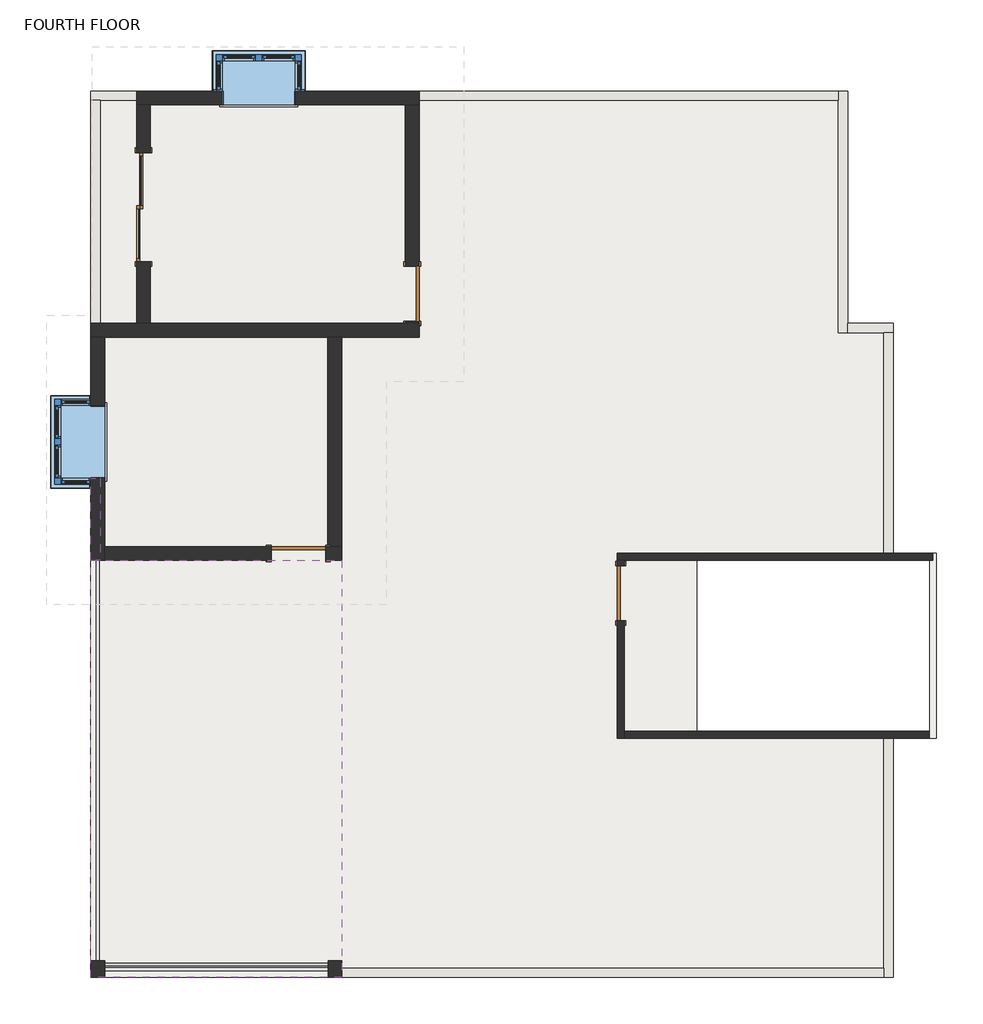
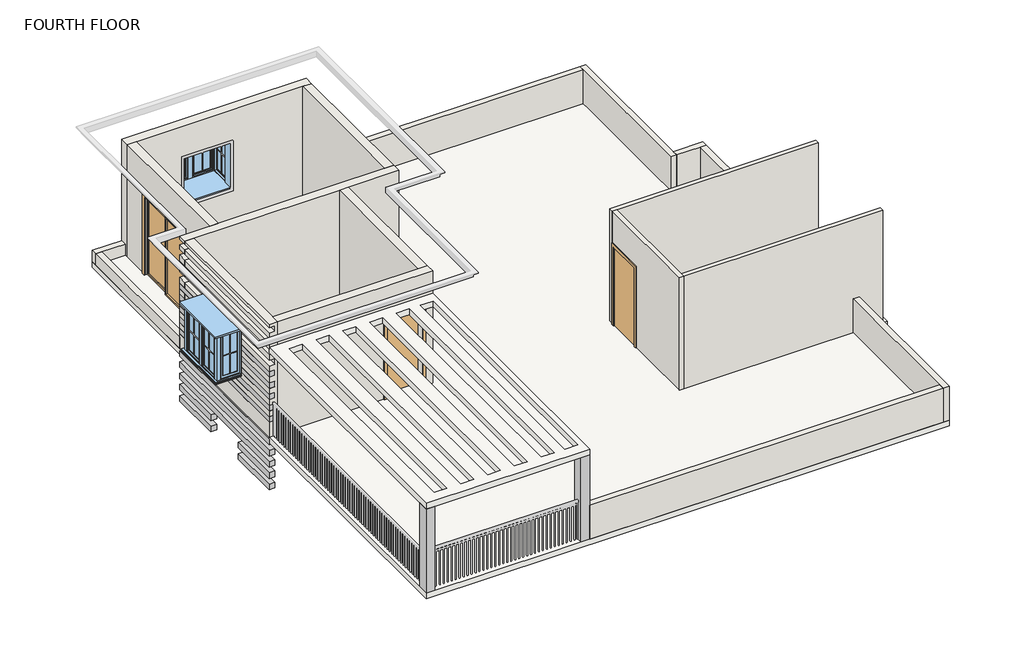
# One storey, part 1 of 2: 18 walls, 10 proxies, 4 doors, 2 columns, 2 slabs, 2 windows.
"""IFC4 building model written with IfcOpenShell, lengths in millimetres."""

from ifc_helpers import new_model, si_unit, frame, origin, place, context, project, spatial, polyline, outline, extrude, faceted_brep, transform, mapped, element, save
from components import door_d4d75d1e, door_0ca8825f, door_e5f9f3c4, window_bay_casement_box_90_degree_angle_4_x4_x2_07b705a1

model = new_model("IFC4")

# Units and contexts
model_context = context("Model", 3, world=origin())
ifc_project = project(units=[si_unit("LENGTHUNIT", "METRE", prefix="MILLI")], contexts=[model_context])

# Site, building, storey
site = spatial("IfcSite", under=ifc_project)
building = spatial("IfcBuilding", under=site)
storey = spatial("IfcBuildingStorey", under=building, Name="FOURTH FLOOR", Elevation=12801.6)

# Proxies
placement = place(None, origin())
element("IfcBuildingElementProxy", 1, Name="Reveal", ObjectType="Reveal", at=placement, inside=storey, context=model_context, shape_type="SweptSolid", body=[
    extrude(outline(polyline([(-7008.3415084, 1592.333346), (-6855.9415084, 1592.333346), (-6855.9415084, 220.733346), (-7008.3415084, 220.733346), (-7008.3415084, 1592.333346)])), frame((0.0, 0.0, 11379.2), z_axis=(0.0, 0.0, 1.0), x_axis=(1.0, 0.0, 0.0)), (0.0, 0.0, 1.0), 152.4),
    extrude(outline(polyline([(-7008.3415084, 4183.133346), (-6855.9415084, 4183.133346), (-6855.9415084, 2811.533346), (-7008.3415084, 2811.533346), (-7008.3415084, 4183.133346)])), frame((0.0, 0.0, 11379.2), z_axis=(0.0, 0.0, 1.0), x_axis=(1.0, 0.0, 0.0)), (0.0, 0.0, 1.0), 152.4),
])
element("IfcBuildingElementProxy", 2, Name="Reveal", ObjectType="Reveal", at=placement, inside=storey, context=model_context, shape_type="SweptSolid", body=[
    extrude(outline(polyline([(-7008.3415084, 1592.333346), (-6855.9415084, 1592.333346), (-6855.9415084, 220.733346), (-7008.3415084, 220.733346), (-7008.3415084, 1592.333346)])), frame((0.0, 0.0, 11684.0), z_axis=(0.0, 0.0, 1.0), x_axis=(1.0, 0.0, 0.0)), (0.0, 0.0, 1.0), 152.4),
    extrude(outline(polyline([(-7008.3415084, 4183.133346), (-6855.9415084, 4183.133346), (-6855.9415084, 2811.533346), (-7008.3415084, 2811.533346), (-7008.3415084, 4183.133346)])), frame((0.0, 0.0, 11684.0), z_axis=(0.0, 0.0, 1.0), x_axis=(1.0, 0.0, 0.0)), (0.0, 0.0, 1.0), 152.4),
])
element("IfcBuildingElementProxy", 3, Name="Reveal", ObjectType="Reveal", at=placement, inside=storey, context=model_context, shape_type="SweptSolid", body=[
    extrude(outline(polyline([(-7008.3415084, 4183.133346), (-6855.9415084, 4183.133346), (-6855.9415084, 220.733346), (-7008.3415084, 220.733346), (-7008.3415084, 4183.133346)])), frame((0.0, 0.0, 11988.8), z_axis=(0.0, 0.0, 1.0), x_axis=(1.0, 0.0, 0.0)), (0.0, 0.0, 1.0), 152.4),
])
element("IfcBuildingElementProxy", 4, Name="Reveal", ObjectType="Reveal", at=placement, inside=storey, context=model_context, shape_type="SweptSolid", body=[
    extrude(outline(polyline([(-7008.3415084, 4183.133346), (-6855.9415084, 4183.133346), (-6855.9415084, 220.733346), (-7008.3415084, 220.733346), (-7008.3415084, 4183.133346)])), frame((0.0, 0.0, 12293.6), z_axis=(0.0, 0.0, 1.0), x_axis=(1.0, 0.0, 0.0)), (0.0, 0.0, 1.0), 152.4),
])
element("IfcBuildingElementProxy", 5, Name="Reveal", ObjectType="Reveal", at=placement, inside=storey, context=model_context, shape_type="SweptSolid", body=[
    extrude(outline(polyline([(-7008.3415084, 4183.133346), (-6855.9415084, 4183.133346), (-6855.9415084, 220.733346), (-7008.3415084, 220.733346), (-7008.3415084, 4183.133346)])), frame((0.0, 0.0, 12598.4), z_axis=(0.0, 0.0, 1.0), x_axis=(1.0, 0.0, 0.0)), (0.0, 0.0, 1.0), 152.4),
])
element("IfcBuildingElementProxy", 6, Name="Reveal", ObjectType="Reveal", at=placement, inside=storey, context=model_context, shape_type="SweptSolid", body=[
    extrude(outline(polyline([(-7008.3415084, 4183.133346), (-6855.9415084, 4183.133346), (-6855.9415084, 220.733346), (-7008.3415084, 220.733346), (-7008.3415084, 4183.133346)])), frame((0.0, 0.0, 13208.0), z_axis=(0.0, 0.0, 1.0), x_axis=(1.0, 0.0, 0.0)), (0.0, 0.0, 1.0), 152.4),
])
element("IfcBuildingElementProxy", 7, Name="Reveal", ObjectType="Reveal", at=placement, inside=storey, context=model_context, shape_type="SweptSolid", body=[
    extrude(outline(polyline([(-7008.3415084, 4183.133346), (-6855.9415084, 4183.133346), (-6855.9415084, 220.733346), (-7008.3415084, 220.733346), (-7008.3415084, 4183.133346)])), frame((0.0, 0.0, 13512.8), z_axis=(0.0, 0.0, 1.0), x_axis=(1.0, 0.0, 0.0)), (0.0, 0.0, 1.0), 152.4),
])
element("IfcBuildingElementProxy", 8, Name="Reveal", ObjectType="Reveal", at=placement, inside=storey, context=model_context, shape_type="SweptSolid", body=[
    extrude(outline(polyline([(-7008.3415084, 1592.333346), (-6855.9415084, 1592.333346), (-6855.9415084, 220.733346), (-7008.3415084, 220.733346), (-7008.3415084, 1592.333346)])), frame((0.0, 0.0, 13817.6), z_axis=(0.0, 0.0, 1.0), x_axis=(1.0, 0.0, 0.0)), (0.0, 0.0, 1.0), 152.4),
    extrude(outline(polyline([(-7008.3415084, 4183.133346), (-6855.9415084, 4183.133346), (-6855.9415084, 2811.533346), (-7008.3415084, 2811.533346), (-7008.3415084, 4183.133346)])), frame((0.0, 0.0, 13817.6), z_axis=(0.0, 0.0, 1.0), x_axis=(1.0, 0.0, 0.0)), (0.0, 0.0, 1.0), 152.4),
])
element("IfcBuildingElementProxy", 9, Name="Reveal", ObjectType="Reveal", at=placement, inside=storey, context=model_context, shape_type="SweptSolid", body=[
    extrude(outline(polyline([(-7008.3415084, 1592.333346), (-6855.9415084, 1592.333346), (-6855.9415084, 220.733346), (-7008.3415084, 220.733346), (-7008.3415084, 1592.333346)])), frame((0.0, 0.0, 14122.4), z_axis=(0.0, 0.0, 1.0), x_axis=(1.0, 0.0, 0.0)), (0.0, 0.0, 1.0), 152.4),
    extrude(outline(polyline([(-7008.3415084, 4183.133346), (-6855.9415084, 4183.133346), (-6855.9415084, 2811.533346), (-7008.3415084, 2811.533346), (-7008.3415084, 4183.133346)])), frame((0.0, 0.0, 14122.4), z_axis=(0.0, 0.0, 1.0), x_axis=(1.0, 0.0, 0.0)), (0.0, 0.0, 1.0), 152.4),
])
element("IfcBuildingElementProxy", 10, Name="Reveal", ObjectType="Reveal", at=placement, inside=storey, context=model_context, shape_type="SweptSolid", body=[
    extrude(outline(polyline([(-7008.3415084, 1592.333346), (-6855.9415084, 1592.333346), (-6855.9415084, 220.733346), (-7008.3415084, 220.733346), (-7008.3415084, 1592.333346)])), frame((0.0, 0.0, 14427.2), z_axis=(0.0, 0.0, 1.0), x_axis=(1.0, 0.0, 0.0)), (0.0, 0.0, 1.0), 152.4),
    extrude(outline(polyline([(-7008.3415084, 4183.133346), (-6855.9415084, 4183.133346), (-6855.9415084, 2811.533346), (-7008.3415084, 2811.533346), (-7008.3415084, 4183.133346)])), frame((0.0, 0.0, 14427.2), z_axis=(0.0, 0.0, 1.0), x_axis=(1.0, 0.0, 0.0)), (0.0, 0.0, 1.0), 152.4),
])

# Columns
element("IfcColumn", 11, ObjectType="Rectangular Column : 9\"x11\"", at=placement, inside=storey, context=model_context, shape_type="SweptSolid", body=[
    extrude(outline(polyline([(-6779.7415084, -6472.166654), (-6779.7415084, -6751.566654), (-7008.3415084, -6751.566654), (-7008.3415084, -6472.166654), (-6779.7415084, -6472.166654)])), frame((0.0, 0.0, 12801.6), z_axis=(0.0, 0.0, 1.0), x_axis=(1.0, 0.0, 0.0)), (0.0, 0.0, 1.0), 2286.0),
])
element("IfcColumn", 12, ObjectType="Rectangular Column : 9\"x11\"", at=placement, inside=storey, context=model_context, shape_type="Brep", body=[
    faceted_brep([(-3040.3749541, -6751.566654, 12801.6), (-3040.3749541, -6472.166654, 12801.6), (-2811.7749541, -6472.166654, 12801.6), (-2811.7749541, -6599.166654, 12801.6), (-2817.3415084, -6599.166654, 12801.6), (-2817.3415084, -6751.566654, 12801.6), (-2811.7749541, -6472.166654, 15087.6), (-2811.7749541, -6751.566654, 15087.6), (-2811.7749541, -6751.566654, 13716.0), (-2811.7749541, -6599.166654, 13716.0), (-3040.3749541, -6751.566654, 15087.6), (-2817.3415084, -6751.566654, 13716.0), (-3040.3749541, -6472.166654, 15087.6), (-2817.3415084, -6599.166654, 13716.0)], [[[0, 1, 2, 3, 4, 5]], [[6, 7, 8, 9, 3, 2]], [[7, 10, 0, 5, 11, 8]], [[1, 0, 10, 12]], [[2, 1, 12, 6]], [[7, 6, 12, 10]], [[13, 4, 3, 9]], [[4, 13, 11, 5]], [[11, 13, 9, 8]]]),
])

# Doors
door_shape = door_d4d75d1e(model_context)
element("IfcDoor", 13, ObjectType="Door-Double-Sliding : 72\" x 84\"", at=placement, inside=storey, context=model_context, shape_type="MappedRepresentation", body=[
    mapped(door_shape, transform((-6005.0415084, 6126.233346, 12801.6), x_axis=(0.0, 1.0, 0.0), y_axis=(-1.0, 0.0, 0.0), z_axis=(0.0, 0.0, 1.0))),
])
door_2_shape = door_0ca8825f(model_context)
element("IfcDoor", 14, ObjectType="Single-Flush : 36\" x 84\"", at=placement, inside=storey, context=model_context, shape_type="MappedRepresentation", body=[
    mapped(door_2_shape, transform((-3541.2415084, 335.033346, 12801.6), x_axis=(1.0, 0.0, 0.0), y_axis=(0.0, 1.0, 0.0), z_axis=(0.0, 0.0, 1.0))),
])
element("IfcDoor", 15, ObjectType="Single-Flush : 36\" x 84\"", at=placement, inside=storey, context=model_context, shape_type="MappedRepresentation", body=[
    mapped(door_2_shape, transform((-1636.2415084, 4678.433346, 12801.6), x_axis=(0.0, -1.0, 0.0), y_axis=(1.0, 0.0, 0.0), z_axis=(0.0, 0.0, 1.0))),
])
door_3_shape = door_e5f9f3c4(model_context)
element("IfcDoor", 16, ObjectType="Single-Flush : 36\" x 84\"", at=placement, inside=storey, context=model_context, shape_type="MappedRepresentation", body=[
    mapped(door_3_shape, transform((1849.1250459, -329.176654, 12801.6), x_axis=(0.0, 1.0, 0.0), y_axis=(-1.0, 0.0, 0.0), z_axis=(0.0, 0.0, 1.0))),
])

# Slabs
element("IfcSlab", 17, ObjectType="6\"", at=placement, inside=storey, context=model_context, shape_type="SweptSolid", body=[
    extrude(outline(polyline([(-7008.3415084, -6751.566654), (-7008.3415084, 220.733346), (-7008.3415084, 8069.333346), (5640.8584916, 8069.333346), (5640.8584916, 4183.133346), (6402.8584916, 4183.133346), (6402.8584916, 337.573346), (7125.9750459, 337.573346), (7125.9750459, -2753.606654), (6402.8584916, -2753.606654), (6402.8584916, -6751.566654), (-7008.3415084, -6751.566654)]), holes=[polyline([(7009.1350459, 220.733346), (3126.2584916, 220.733346), (3126.2584916, -2636.766654), (7009.1350459, -2636.766654), (7009.1350459, 220.733346)])]), frame((0.0, 0.0, 12649.2), z_axis=(0.0, 0.0, 1.0), x_axis=(1.0, 0.0, 0.0)), (0.0, 0.0, 1.0), 152.4),
])
element("IfcSlab", 18, ObjectType="6\"", at=placement, inside=storey, context=model_context, shape_type="SweptSolid", body=[
    extrude(outline(polyline([(-7008.3415084, -6751.566654), (-7008.3415084, 220.733346), (-2817.3415084, 220.733346), (-2817.3415084, -6751.566654), (-7008.3415084, -6751.566654)]), holes=[polyline([(-6310.7833787, -45.9532972), (-6640.9833787, -45.9532972), (-6640.9833787, -6472.166654), (-6310.7833787, -6472.166654), (-6310.7833787, -45.9532972)]), polyline([(-5624.9833787, -45.9532972), (-5955.1833787, -45.9532972), (-5955.1833787, -6472.166654), (-5624.9833787, -6472.166654), (-5624.9833787, -45.9532972)]), polyline([(-4939.1833787, -45.9532972), (-5269.3833787, -45.9532972), (-5269.3833787, -6472.166654), (-4939.1833787, -6472.166654), (-4939.1833787, -45.9532972)]), polyline([(-4253.3833787, -45.9532972), (-4583.5833787, -45.9532972), (-4583.5833787, -6472.166654), (-4253.3833787, -6472.166654), (-4253.3833787, -45.9532972)]), polyline([(-3567.5833787, -45.9532972), (-3897.7833787, -45.9532972), (-3897.7833787, -6472.166654), (-3567.5833787, -6472.166654), (-3567.5833787, -45.9532972)]), polyline([(-2957.9833787, -45.9532972), (-3288.1833787, -45.9532972), (-3288.1833787, -6472.166654), (-2957.9833787, -6472.166654), (-2957.9833787, -45.9532972)])]), frame((0.0, 0.0, 15087.6), z_axis=(0.0, 0.0, 1.0), x_axis=(1.0, 0.0, 0.0)), (0.0, 0.0, 1.0), 152.4),
])

# Walls
element("IfcWall", 19, ObjectType="4.5\"", at=placement, inside=storey, context=model_context, shape_type="Brep", body=[
    faceted_brep([(7068.8250459, 337.573346, 12801.6), (6402.8584916, 337.573346, 12801.6), (6250.4584916, 337.573346, 12801.6), (1791.9750459, 337.573346, 12801.6), (1791.9750459, 337.573346, 15849.6), (7068.8250459, 337.573346, 15849.6), (7068.8250459, 223.273346, 12801.6), (7068.8250459, 223.273346, 15849.6), (1906.2750459, 223.273346, 15849.6), (1791.9750459, 223.273346, 15849.6), (1791.9750459, 223.273346, 12801.6), (1906.2750459, 223.273346, 12801.6)], [[[0, 1, 2, 3, 4, 5]], [[6, 7, 8, 9, 10, 11]], [[3, 2, 1, 0, 6, 11, 10]], [[5, 4, 9, 8, 7]], [[0, 5, 7, 6]], [[4, 3, 10, 9]]]),
])
element("IfcWall", 20, ObjectType="4.5\"", at=placement, inside=storey, context=model_context, shape_type="Brep", body=[
    faceted_brep([(1791.9750459, 223.273346, 12801.6), (1791.9750459, 128.023346, 12801.6), (1791.9750459, 128.023346, 14935.2), (1791.9750459, -786.376654, 14935.2), (1791.9750459, -786.376654, 12801.6), (1791.9750459, -2753.606654, 12801.6), (1791.9750459, -2753.606654, 15849.6), (1791.9750459, 223.273346, 15849.6), (1906.2750459, 128.023346, 14935.2), (1906.2750459, 128.023346, 12801.6), (1906.2750459, 223.273346, 12801.6), (1906.2750459, 223.273346, 15849.6), (1906.2750459, -2639.306654, 15849.6), (1906.2750459, -2753.606654, 15849.6), (1906.2750459, -2753.606654, 12801.6), (1906.2750459, -2639.306654, 12801.6), (1906.2750459, -786.376654, 12801.6), (1906.2750459, -786.376654, 14935.2)], [[[0, 1, 2, 3, 4, 5, 6, 7]], [[8, 9, 10, 11, 12, 13, 14, 15, 16, 17]], [[10, 9, 1, 0]], [[16, 15, 14, 5, 4]], [[7, 6, 13, 12, 11]], [[0, 7, 11, 10]], [[6, 5, 14, 13]], [[2, 1, 9, 8]], [[3, 2, 8, 17]], [[4, 3, 17, 16]]]),
])
element("IfcWall", 21, ObjectType="4.5\"", at=placement, inside=storey, context=model_context, shape_type="Brep", body=[
    faceted_brep([(1906.2750459, -2753.606654, 12801.6), (6250.4584916, -2753.606654, 12801.6), (6402.8584916, -2753.606654, 12801.6), (7009.1350459, -2753.606654, 12801.6), (7009.1350459, -2753.606654, 15849.6), (1906.2750459, -2753.606654, 15849.6), (1906.2750459, -2639.306654, 12801.6), (1906.2750459, -2639.306654, 15849.6), (7009.1350459, -2639.306654, 15849.6), (7009.1350459, -2639.306654, 12801.6)], [[[0, 1, 2, 3, 4, 5]], [[6, 7, 8, 9]], [[3, 2, 1, 0, 6, 9]], [[5, 4, 8, 7]], [[0, 5, 7, 6]], [[4, 3, 9, 8]]]),
])
element("IfcWall", 22, ObjectType="6\"", at=placement, inside=storey, context=model_context, shape_type="Brep", body=[
    faceted_brep([(6250.4584916, -2753.606654, 12801.6), (6250.4584916, -6599.166654, 12801.6), (6250.4584916, -6751.566654, 12801.6), (6250.4584916, -6751.566654, 13716.0), (6250.4584916, -6599.166654, 13716.0), (6250.4584916, -2753.606654, 13716.0), (6402.8584916, -2753.606654, 12801.6), (6402.8584916, -2753.606654, 13716.0), (6402.8584916, -6751.566654, 13716.0), (6402.8584916, -6751.566654, 12801.6)], [[[0, 1, 2, 3, 4, 5]], [[6, 7, 8, 9]], [[2, 1, 0, 6, 9]], [[5, 4, 3, 8, 7]], [[0, 5, 7, 6]], [[3, 2, 9, 8]]]),
])
element("IfcWall", 23, ObjectType="6\"", at=placement, inside=storey, context=model_context, shape_type="Brep", body=[
    faceted_brep([(6250.4584916, -6599.166654, 12801.6), (-2811.7749541, -6599.166654, 12801.6), (-2817.3415084, -6599.166654, 12801.6), (-2817.3415084, -6599.166654, 13716.0), (-2811.7749541, -6599.166654, 13716.0), (6250.4584916, -6599.166654, 13716.0), (6250.4584916, -6751.566654, 12801.6), (6250.4584916, -6751.566654, 13716.0), (-2811.7749541, -6751.566654, 13716.0), (-2817.3415084, -6751.566654, 13716.0), (-2817.3415084, -6751.566654, 12801.6)], [[[0, 1, 2, 3, 4, 5]], [[6, 7, 8, 9, 10]], [[2, 1, 0, 6, 10]], [[3, 2, 10, 9]], [[5, 4, 3, 9, 8, 7]], [[0, 5, 7, 6]]]),
])
element("IfcWall", 24, ObjectType="6\"", at=placement, inside=storey, context=model_context, shape_type="Brep", body=[
    faceted_brep([(5488.4584916, 8069.333346, 12801.6), (5488.4584916, 7916.933346, 12801.6), (5488.4584916, 4030.733346, 12801.6), (5488.4584916, 4030.733346, 13716.0), (5488.4584916, 7916.933346, 13716.0), (5488.4584916, 8069.333346, 13716.0), (5640.8584916, 8069.333346, 12801.6), (5640.8584916, 8069.333346, 13716.0), (5640.8584916, 4183.133346, 13716.0), (5640.8584916, 4030.733346, 13716.0), (5640.8584916, 4030.733346, 12801.6), (5640.8584916, 4183.133346, 12801.6)], [[[0, 1, 2, 3, 4, 5]], [[6, 7, 8, 9, 10, 11]], [[2, 1, 0, 6, 11, 10]], [[5, 4, 3, 9, 8, 7]], [[3, 2, 10, 9]], [[0, 5, 7, 6]]]),
])
element("IfcWall", 25, ObjectType="6\"", at=placement, inside=storey, context=model_context, shape_type="Brep", body=[
    faceted_brep([(5640.8584916, 4030.733346, 12801.6), (6250.4584916, 4030.733346, 12801.6), (6402.8584916, 4030.733346, 12801.6), (6402.8584916, 4030.733346, 13716.0), (6250.4584916, 4030.733346, 13716.0), (5640.8584916, 4030.733346, 13716.0), (5640.8584916, 4183.133346, 12801.6), (5640.8584916, 4183.133346, 13716.0), (6402.8584916, 4183.133346, 13716.0), (6402.8584916, 4183.133346, 12801.6)], [[[0, 1, 2, 3, 4, 5]], [[6, 7, 8, 9]], [[2, 1, 0, 6, 9]], [[5, 4, 3, 8, 7]], [[0, 5, 7, 6]], [[3, 2, 9, 8]]]),
])
element("IfcWall", 26, ObjectType="6\"", at=placement, inside=storey, context=model_context, shape_type="SweptSolid", body=[
    extrude(outline(polyline([(6250.4584916, 337.573346), (6250.4584916, 4030.733346), (6402.8584916, 4030.733346), (6402.8584916, 337.573346), (6250.4584916, 337.573346)])), frame((0.0, 0.0, 12801.6), z_axis=(0.0, 0.0, 1.0), x_axis=(1.0, 0.0, 0.0)), (0.0, 0.0, 1.0), 914.4),
])
element("IfcWall", 27, ObjectType="6\"", at=placement, inside=storey, context=model_context, shape_type="SweptSolid", body=[
    extrude(outline(polyline([(-1521.9415084, 8069.333346), (5488.4584916, 8069.333346), (5488.4584916, 7916.933346), (-1521.9415084, 7916.933346), (-1521.9415084, 8069.333346)])), frame((0.0, 0.0, 12801.6), z_axis=(0.0, 0.0, 1.0), x_axis=(1.0, 0.0, 0.0)), (0.0, 0.0, 1.0), 914.4),
])
element("IfcWall", 28, ObjectType="6\"", at=placement, inside=storey, context=model_context, shape_type="Brep", body=[
    faceted_brep([(-6246.3415084, 8069.333346, 12801.6), (-7008.3415084, 8069.333346, 12801.6), (-7008.3415084, 8069.333346, 13106.4), (-6246.3415084, 8069.333346, 13106.4), (-6246.3415084, 7916.933346, 12801.6), (-6246.3415084, 7916.933346, 13106.4), (-6855.9415084, 7916.933346, 13106.4), (-7008.3415084, 7916.933346, 13106.4), (-7008.3415084, 7916.933346, 12801.6), (-6855.9415084, 7916.933346, 12801.6)], [[[0, 1, 2, 3]], [[4, 5, 6, 7, 8, 9]], [[1, 0, 4, 9, 8]], [[3, 2, 7, 6, 5]], [[2, 1, 8, 7]], [[0, 3, 5, 4]]]),
])
element("IfcWall", 29, ObjectType="6\"", at=placement, inside=storey, context=model_context, shape_type="SweptSolid", body=[
    extrude(outline(polyline([(-7008.3415084, 4183.133346), (-7008.3415084, 7916.933346), (-6855.9415084, 7916.933346), (-6855.9415084, 4183.133346), (-7008.3415084, 4183.133346)])), frame((0.0, 0.0, 12801.6), z_axis=(0.0, 0.0, 1.0), x_axis=(1.0, 0.0, 0.0)), (0.0, 0.0, 1.0), 304.8),
])
element("IfcWall", 30, ObjectType="9\"", at=placement, inside=storey, context=model_context, shape_type="Brep", body=[
    faceted_brep([(-1521.9415084, 8069.333346, 12801.6), (-6246.3415084, 8069.333346, 12801.6), (-6246.3415084, 8069.333346, 13106.4), (-6246.3415084, 8069.333346, 15849.6), (-1521.9415084, 8069.333346, 15849.6), (-1521.9415084, 8069.333346, 13716.0), (-3592.0415084, 8069.333346, 14986.0), (-4811.2415084, 8069.333346, 14986.0), (-4811.2415084, 8069.333346, 13716.0), (-3592.0415084, 8069.333346, 13716.0), (-1521.9415084, 7840.733346, 12801.6), (-1521.9415084, 7840.733346, 15849.6), (-1750.5415084, 7840.733346, 15849.6), (-6017.7415084, 7840.733346, 15849.6), (-6246.3415084, 7840.733346, 15849.6), (-6246.3415084, 7840.733346, 12801.6), (-6017.7415084, 7840.733346, 12801.6), (-1750.5415084, 7840.733346, 12801.6), (-3592.0415084, 7840.733346, 14986.0), (-3592.0415084, 7840.733346, 13716.0), (-4811.2415084, 7840.733346, 13716.0), (-4811.2415084, 7840.733346, 14986.0), (-1521.9415084, 7916.933346, 12801.6), (-6246.3415084, 7916.933346, 12801.6)], [[[0, 1, 2, 3, 4, 5], [6, 7, 8, 9]], [[10, 11, 12, 13, 14, 15, 16, 17], [18, 19, 20, 21]], [[1, 0, 22, 10, 17, 16, 15, 23]], [[4, 3, 14, 13, 12, 11]], [[0, 5, 4, 11, 10, 22]], [[19, 18, 6, 9]], [[20, 19, 9, 8]], [[21, 20, 8, 7]], [[18, 21, 7, 6]], [[1, 23, 15, 14, 3, 2]]]),
])
element("IfcWall", 31, ObjectType="9\"", at=placement, inside=storey, context=model_context, shape_type="SweptSolid", body=[
    extrude(outline(polyline([(7840.733346, 12801.6), (7040.633346, 12801.6), (7040.633346, 14935.2), (5211.833346, 14935.2), (5211.833346, 12801.6), (4183.133346, 12801.6), (4183.133346, 15849.6), (7840.733346, 15849.6), (7840.733346, 12801.6)])), frame((-6246.3415084, 0.0, 0.0), z_axis=(1.0, 0.0, 0.0), x_axis=(0.0, 1.0, 0.0)), (0.0, 0.0, 1.0), 228.6),
])
element("IfcWall", 32, ObjectType="9\"", at=placement, inside=storey, context=model_context, shape_type="SweptSolid", body=[
    extrude(outline(polyline([(4221.233346, 14935.2), (4221.233346, 12801.6), (4183.133346, 12801.6), (4183.133346, 15849.6), (7840.733346, 15849.6), (7840.733346, 12801.6), (5135.633346, 12801.6), (5135.633346, 14935.2), (4221.233346, 14935.2)])), frame((-1750.5415084, 0.0, 0.0), z_axis=(1.0, 0.0, 0.0), x_axis=(0.0, 1.0, 0.0)), (0.0, 0.0, 1.0), 228.6),
])
element("IfcWall", 33, ObjectType="9\"", at=placement, inside=storey, context=model_context, shape_type="Brep", body=[
    faceted_brep([(-1521.9415084, 4183.133346, 12801.6), (-1750.5415084, 4183.133346, 12801.6), (-6017.7415084, 4183.133346, 12801.6), (-6246.3415084, 4183.133346, 12801.6), (-6855.9415084, 4183.133346, 12801.6), (-7008.3415084, 4183.133346, 12801.6), (-7008.3415084, 4183.133346, 13106.4), (-7008.3415084, 4183.133346, 13208.0), (-6855.9415084, 4183.133346, 13208.0), (-6855.9415084, 4183.133346, 13360.4), (-7008.3415084, 4183.133346, 13360.4), (-7008.3415084, 4183.133346, 13512.8), (-6855.9415084, 4183.133346, 13512.8), (-6855.9415084, 4183.133346, 13665.2), (-7008.3415084, 4183.133346, 13665.2), (-7008.3415084, 4183.133346, 13817.6), (-6855.9415084, 4183.133346, 13817.6), (-6855.9415084, 4183.133346, 13970.0), (-7008.3415084, 4183.133346, 13970.0), (-7008.3415084, 4183.133346, 14122.4), (-6855.9415084, 4183.133346, 14122.4), (-6855.9415084, 4183.133346, 14274.8), (-7008.3415084, 4183.133346, 14274.8), (-7008.3415084, 4183.133346, 14427.2), (-6855.9415084, 4183.133346, 14427.2), (-6855.9415084, 4183.133346, 14579.6), (-7008.3415084, 4183.133346, 14579.6), (-7008.3415084, 4183.133346, 14732.0), (-6855.9415084, 4183.133346, 14732.0), (-6855.9415084, 4183.133346, 14884.4), (-7008.3415084, 4183.133346, 14884.4), (-7008.3415084, 4183.133346, 15036.8), (-6855.9415084, 4183.133346, 15036.8), (-6855.9415084, 4183.133346, 15189.2), (-7008.3415084, 4183.133346, 15189.2), (-7008.3415084, 4183.133346, 15341.6), (-6855.9415084, 4183.133346, 15341.6), (-6855.9415084, 4183.133346, 15494.0), (-7008.3415084, 4183.133346, 15494.0), (-7008.3415084, 4183.133346, 15621.0), (-6855.9415084, 4183.133346, 15621.0), (-6855.9415084, 4183.133346, 15773.4), (-7008.3415084, 4183.133346, 15773.4), (-7008.3415084, 4183.133346, 15849.6), (-6246.3415084, 4183.133346, 15849.6), (-6017.7415084, 4183.133346, 15849.6), (-1750.5415084, 4183.133346, 15849.6), (-1521.9415084, 4183.133346, 15849.6), (-7008.3415084, 3954.533346, 12801.6), (-6779.7415084, 3954.533346, 12801.6), (-3045.9415084, 3954.533346, 12801.6), (-2817.3415084, 3954.533346, 12801.6), (-1521.9415084, 3954.533346, 12801.6), (-1521.9415084, 3954.533346, 15849.6), (-2817.3415084, 3954.533346, 15849.6), (-3045.9415084, 3954.533346, 15849.6), (-6779.7415084, 3954.533346, 15849.6), (-7008.3415084, 3954.533346, 15849.6), (-7008.3415084, 3954.533346, 15773.4), (-6855.9415084, 3954.533346, 15773.4), (-6855.9415084, 3954.533346, 15621.0), (-7008.3415084, 3954.533346, 15621.0), (-7008.3415084, 3954.533346, 15494.0), (-6855.9415084, 3954.533346, 15494.0), (-6855.9415084, 3954.533346, 15341.6), (-7008.3415084, 3954.533346, 15341.6), (-7008.3415084, 3954.533346, 15189.2), (-6855.9415084, 3954.533346, 15189.2), (-6855.9415084, 3954.533346, 15036.8), (-7008.3415084, 3954.533346, 15036.8), (-7008.3415084, 3954.533346, 14884.4), (-6855.9415084, 3954.533346, 14884.4), (-6855.9415084, 3954.533346, 14732.0), (-7008.3415084, 3954.533346, 14732.0), (-7008.3415084, 3954.533346, 14579.6), (-6855.9415084, 3954.533346, 14579.6), (-6855.9415084, 3954.533346, 14427.2), (-7008.3415084, 3954.533346, 14427.2), (-7008.3415084, 3954.533346, 14274.8), (-6855.9415084, 3954.533346, 14274.8), (-6855.9415084, 3954.533346, 14122.4), (-7008.3415084, 3954.533346, 14122.4), (-7008.3415084, 3954.533346, 13970.0), (-6855.9415084, 3954.533346, 13970.0), (-6855.9415084, 3954.533346, 13817.6), (-7008.3415084, 3954.533346, 13817.6), (-7008.3415084, 3954.533346, 13665.2), (-6855.9415084, 3954.533346, 13665.2), (-6855.9415084, 3954.533346, 13512.8), (-7008.3415084, 3954.533346, 13512.8), (-7008.3415084, 3954.533346, 13360.4), (-6855.9415084, 3954.533346, 13360.4), (-6855.9415084, 3954.533346, 13208.0), (-7008.3415084, 3954.533346, 13208.0)], [[[0, 1, 2, 3, 4, 5, 6, 7, 8, 9, 10, 11, 12, 13, 14, 15, 16, 17, 18, 19, 20, 21, 22, 23, 24, 25, 26, 27, 28, 29, 30, 31, 32, 33, 34, 35, 36, 37, 38, 39, 40, 41, 42, 43, 44, 45, 46, 47]], [[48, 49, 50, 51, 52, 53, 54, 55, 56, 57, 58, 59, 60, 61, 62, 63, 64, 65, 66, 67, 68, 69, 70, 71, 72, 73, 74, 75, 76, 77, 78, 79, 80, 81, 82, 83, 84, 85, 86, 87, 88, 89, 90, 91, 92, 93]], [[5, 4, 3, 2, 1, 0, 52, 51, 50, 49, 48]], [[47, 46, 45, 44, 43, 57, 56, 55, 54, 53]], [[0, 47, 53, 52]], [[5, 48, 93, 7, 6]], [[57, 43, 42, 58]], [[34, 66, 65, 35]], [[69, 31, 30, 70]], [[73, 27, 26, 74]], [[77, 23, 22, 78]], [[81, 19, 18, 82]], [[85, 15, 14, 86]], [[89, 11, 10, 90]], [[38, 62, 61, 39]], [[33, 67, 66, 34]], [[67, 33, 32, 68]], [[68, 32, 31, 69]], [[29, 71, 70, 30]], [[71, 29, 28, 72]], [[72, 28, 27, 73]], [[25, 75, 74, 26]], [[75, 25, 24, 76]], [[76, 24, 23, 77]], [[21, 79, 78, 22]], [[79, 21, 20, 80]], [[80, 20, 19, 81]], [[17, 83, 82, 18]], [[83, 17, 16, 84]], [[84, 16, 15, 85]], [[13, 87, 86, 14]], [[87, 13, 12, 88]], [[88, 12, 11, 89]], [[9, 91, 90, 10]], [[91, 9, 8, 92]], [[92, 8, 7, 93]], [[37, 63, 62, 38]], [[63, 37, 36, 64]], [[64, 36, 35, 65]], [[41, 59, 58, 42]], [[59, 41, 40, 60]], [[60, 40, 39, 61]]]),
])
element("IfcWall", 34, ObjectType="9\"", at=placement, inside=storey, context=model_context, shape_type="Brep", body=[
    faceted_brep([(-7008.3415084, 3954.533346, 12801.6), (-7008.3415084, 220.733346, 12801.6), (-7008.3415084, 220.733346, 13208.0), (-7008.3415084, 3954.533346, 13208.0), (-7008.3415084, 220.733346, 15849.6), (-7008.3415084, 3954.533346, 15849.6), (-7008.3415084, 3954.533346, 15773.4), (-7008.3415084, 220.733346, 15773.4), (-7008.3415084, 1592.333346, 13716.0), (-7008.3415084, 2811.533346, 13716.0), (-7008.3415084, 2811.533346, 13817.6), (-7008.3415084, 3954.533346, 13817.6), (-7008.3415084, 3954.533346, 13665.2), (-7008.3415084, 220.733346, 13665.2), (-7008.3415084, 220.733346, 13817.6), (-7008.3415084, 1592.333346, 13817.6), (-7008.3415084, 2811.533346, 14986.0), (-7008.3415084, 1592.333346, 14986.0), (-7008.3415084, 1592.333346, 14884.4), (-7008.3415084, 220.733346, 14884.4), (-7008.3415084, 220.733346, 15036.8), (-7008.3415084, 3954.533346, 15036.8), (-7008.3415084, 3954.533346, 14884.4), (-7008.3415084, 2811.533346, 14884.4), (-7008.3415084, 3954.533346, 15189.2), (-7008.3415084, 220.733346, 15189.2), (-7008.3415084, 220.733346, 15341.6), (-7008.3415084, 3954.533346, 15341.6), (-7008.3415084, 220.733346, 14732.0), (-7008.3415084, 1592.333346, 14732.0), (-7008.3415084, 1592.333346, 14579.6), (-7008.3415084, 220.733346, 14579.6), (-7008.3415084, 2811.533346, 14732.0), (-7008.3415084, 3954.533346, 14732.0), (-7008.3415084, 3954.533346, 14579.6), (-7008.3415084, 2811.533346, 14579.6), (-7008.3415084, 220.733346, 14427.2), (-7008.3415084, 1592.333346, 14427.2), (-7008.3415084, 1592.333346, 14274.8), (-7008.3415084, 220.733346, 14274.8), (-7008.3415084, 2811.533346, 14427.2), (-7008.3415084, 3954.533346, 14427.2), (-7008.3415084, 3954.533346, 14274.8), (-7008.3415084, 2811.533346, 14274.8), (-7008.3415084, 220.733346, 14122.4), (-7008.3415084, 1592.333346, 14122.4), (-7008.3415084, 1592.333346, 13970.0), (-7008.3415084, 220.733346, 13970.0), (-7008.3415084, 2811.533346, 14122.4), (-7008.3415084, 3954.533346, 14122.4), (-7008.3415084, 3954.533346, 13970.0), (-7008.3415084, 2811.533346, 13970.0), (-7008.3415084, 220.733346, 13512.8), (-7008.3415084, 3954.533346, 13512.8), (-7008.3415084, 3954.533346, 13360.4), (-7008.3415084, 220.733346, 13360.4), (-7008.3415084, 3954.533346, 15494.0), (-7008.3415084, 220.733346, 15494.0), (-7008.3415084, 220.733346, 15621.0), (-7008.3415084, 3954.533346, 15621.0), (-6779.7415084, 220.733346, 12801.6), (-6779.7415084, 449.333346, 12801.6), (-6779.7415084, 3954.533346, 12801.6), (-6779.7415084, 3954.533346, 15849.6), (-6779.7415084, 449.333346, 15849.6), (-6779.7415084, 220.733346, 15849.6), (-6779.7415084, 2811.533346, 14986.0), (-6779.7415084, 2811.533346, 13716.0), (-6779.7415084, 1592.333346, 13716.0), (-6779.7415084, 1592.333346, 14986.0), (-6855.9415084, 220.733346, 15773.4), (-6855.9415084, 220.733346, 15621.0), (-6855.9415084, 220.733346, 15494.0), (-6855.9415084, 220.733346, 15341.6), (-6855.9415084, 220.733346, 15189.2), (-6855.9415084, 220.733346, 15036.8), (-6855.9415084, 220.733346, 14884.4), (-6855.9415084, 220.733346, 14732.0), (-6855.9415084, 220.733346, 14579.6), (-6855.9415084, 220.733346, 14427.2), (-6855.9415084, 220.733346, 14274.8), (-6855.9415084, 220.733346, 14122.4), (-6855.9415084, 220.733346, 13970.0), (-6855.9415084, 220.733346, 13817.6), (-6855.9415084, 220.733346, 13665.2), (-6855.9415084, 220.733346, 13512.8), (-6855.9415084, 220.733346, 13360.4), (-6855.9415084, 220.733346, 13208.0), (-6855.9415084, 2811.533346, 14884.4), (-6855.9415084, 2811.533346, 14732.0), (-6855.9415084, 2811.533346, 14579.6), (-6855.9415084, 2811.533346, 14427.2), (-6855.9415084, 2811.533346, 14274.8), (-6855.9415084, 2811.533346, 14122.4), (-6855.9415084, 2811.533346, 13970.0), (-6855.9415084, 2811.533346, 13817.6), (-6855.9415084, 1592.333346, 13817.6), (-6855.9415084, 1592.333346, 13970.0), (-6855.9415084, 1592.333346, 14122.4), (-6855.9415084, 1592.333346, 14274.8), (-6855.9415084, 1592.333346, 14427.2), (-6855.9415084, 1592.333346, 14579.6), (-6855.9415084, 1592.333346, 14732.0), (-6855.9415084, 1592.333346, 14884.4), (-6855.9415084, 3954.533346, 13208.0), (-6855.9415084, 3954.533346, 13360.4), (-6855.9415084, 3954.533346, 13512.8), (-6855.9415084, 3954.533346, 13665.2), (-6855.9415084, 3954.533346, 13817.6), (-6855.9415084, 3954.533346, 13970.0), (-6855.9415084, 3954.533346, 14122.4), (-6855.9415084, 3954.533346, 14274.8), (-6855.9415084, 3954.533346, 14427.2), (-6855.9415084, 3954.533346, 14579.6), (-6855.9415084, 3954.533346, 14732.0), (-6855.9415084, 3954.533346, 14884.4), (-6855.9415084, 3954.533346, 15036.8), (-6855.9415084, 3954.533346, 15189.2), (-6855.9415084, 3954.533346, 15341.6), (-6855.9415084, 3954.533346, 15494.0), (-6855.9415084, 3954.533346, 15621.0), (-6855.9415084, 3954.533346, 15773.4)], [[[0, 1, 2, 3]], [[4, 5, 6, 7]], [[8, 9, 10, 11, 12, 13, 14, 15]], [[16, 17, 18, 19, 20, 21, 22, 23]], [[24, 25, 26, 27]], [[28, 29, 30, 31]], [[32, 33, 34, 35]], [[36, 37, 38, 39]], [[40, 41, 42, 43]], [[44, 45, 46, 47]], [[48, 49, 50, 51]], [[52, 53, 54, 55]], [[56, 57, 58, 59]], [[60, 61, 62, 63, 64, 65], [66, 67, 68, 69]], [[1, 0, 62, 61, 60]], [[5, 4, 65, 64, 63]], [[1, 60, 65, 4, 7, 70, 71, 58, 57, 72, 73, 26, 25, 74, 75, 20, 19, 76, 77, 28, 31, 78, 79, 36, 39, 80, 81, 44, 47, 82, 83, 14, 13, 84, 85, 52, 55, 86, 87, 2]], [[67, 66, 16, 23, 88, 89, 32, 35, 90, 91, 40, 43, 92, 93, 48, 51, 94, 95, 10, 9]], [[68, 67, 9, 8]], [[69, 68, 8, 15, 96, 97, 46, 45, 98, 99, 38, 37, 100, 101, 30, 29, 102, 103, 18, 17]], [[66, 69, 17, 16]], [[5, 63, 62, 0, 3, 104, 105, 54, 53, 106, 107, 12, 11, 108, 109, 50, 49, 110, 111, 42, 41, 112, 113, 34, 33, 114, 115, 22, 21, 116, 117, 24, 27, 118, 119, 56, 59, 120, 121, 6]], [[117, 74, 25, 24]], [[74, 117, 116, 75]], [[75, 116, 21, 20]], [[103, 76, 19, 18]], [[76, 103, 102, 77]], [[77, 102, 29, 28]], [[115, 88, 23, 22]], [[88, 115, 114, 89]], [[89, 114, 33, 32]], [[101, 78, 31, 30]], [[78, 101, 100, 79]], [[79, 100, 37, 36]], [[113, 90, 35, 34]], [[90, 113, 112, 91]], [[91, 112, 41, 40]], [[99, 80, 39, 38]], [[80, 99, 98, 81]], [[81, 98, 45, 44]], [[111, 92, 43, 42]], [[92, 111, 110, 93]], [[93, 110, 49, 48]], [[97, 82, 47, 46]], [[82, 97, 96, 83]], [[83, 96, 15, 14]], [[109, 94, 51, 50]], [[94, 109, 108, 95]], [[95, 108, 11, 10]], [[107, 84, 13, 12]], [[84, 107, 106, 85]], [[85, 106, 53, 52]], [[105, 86, 55, 54]], [[86, 105, 104, 87]], [[87, 104, 3, 2]], [[119, 72, 57, 56]], [[72, 119, 118, 73]], [[73, 118, 27, 26]], [[121, 70, 7, 6]], [[70, 121, 120, 71]], [[71, 120, 59, 58]]]),
])
element("IfcWall", 35, ObjectType="9\"", at=placement, inside=storey, context=model_context, shape_type="Brep", body=[
    faceted_brep([(-3084.0415084, 220.733346, 14935.2), (-3084.0415084, 220.733346, 12801.6), (-2817.3415084, 220.733346, 12801.6), (-2817.3415084, 220.733346, 15849.6), (-6779.7415084, 220.733346, 15849.6), (-6779.7415084, 220.733346, 12801.6), (-3998.4415084, 220.733346, 12801.6), (-3998.4415084, 220.733346, 14935.2), (-2817.3415084, 449.333346, 12801.6), (-3045.9415084, 449.333346, 12801.6), (-3084.0415084, 449.333346, 12801.6), (-3084.0415084, 449.333346, 14935.2), (-3998.4415084, 449.333346, 14935.2), (-3998.4415084, 449.333346, 12801.6), (-6779.7415084, 449.333346, 12801.6), (-6779.7415084, 449.333346, 15849.6), (-3045.9415084, 449.333346, 15849.6), (-2817.3415084, 449.333346, 15849.6)], [[[0, 1, 2, 3, 4, 5, 6, 7]], [[8, 9, 10, 11, 12, 13, 14, 15, 16, 17]], [[6, 5, 14, 13]], [[2, 1, 10, 9, 8]], [[4, 3, 17, 16, 15]], [[5, 4, 15, 14]], [[3, 2, 8, 17]], [[11, 10, 1, 0]], [[12, 11, 0, 7]], [[13, 12, 7, 6]]]),
])
element("IfcWall", 36, ObjectType="9\"", at=placement, inside=storey, context=model_context, shape_type="SweptSolid", body=[
    extrude(outline(polyline([(-2817.3415084, 3954.533346), (-2817.3415084, 449.333346), (-3045.9415084, 449.333346), (-3045.9415084, 3954.533346), (-2817.3415084, 3954.533346)])), frame((0.0, 0.0, 12801.6), z_axis=(0.0, 0.0, 1.0), x_axis=(1.0, 0.0, 0.0)), (0.0, 0.0, 1.0), 3048.0),
])

# Windows
window_bay_casement_box_90_degree_angle_4_x4_x2_shape = window_bay_casement_box_90_degree_angle_4_x4_x2_07b705a1(model_context)
element("IfcWindow", 37, ObjectType="Window-Bay-Casement-Box-90_Degree_Angle : 4'X4'X2'", at=placement, inside=storey, context=model_context, shape_type="MappedRepresentation", body=[
    mapped(window_bay_casement_box_90_degree_angle_4_x4_x2_shape, transform((-4201.6415084, 7955.033346, 13106.4), x_axis=(1.0, 0.0, 0.0), y_axis=(0.0, 1.0, 0.0), z_axis=(0.0, 0.0, 1.0))),
])
element("IfcWindow", 38, ObjectType="Window-Bay-Casement-Box-90_Degree_Angle : 4'X4'X2'", at=placement, inside=storey, context=model_context, shape_type="MappedRepresentation", body=[
    mapped(window_bay_casement_box_90_degree_angle_4_x4_x2_shape, transform((-6894.0415084, 2201.933346, 13106.4), x_axis=(0.0, 1.0, 0.0), y_axis=(-1.0, 0.0, 0.0), z_axis=(0.0, 0.0, 1.0))),
])

save(model, "model.ifc")

# Revit data of these elements
# Type "Rectangular Column : 9\"x11\""
#   Assembly Code = "B1010200"
#   Depth = 0' - 11"
#   Offset Base = 0' - 0"
#   Offset Top = 0' - 0"
#   Width = 0' - 9"
#   Material = none
# Type "Door-Double-Sliding : 72\" x 84\""
#   Type Mark = "10"
#   Construction Type Id = "opn-d45"
#   Assembly Code = "C1020"
#   Analytic Construction = "Wood frame, double glass door "
#   Thickness = 0' - 2"
#   Thermal Resistance (R) = 1.8150 (h·ft²·°F)/BTU
#   Heat Transfer Coefficient (U) = 0.5510 BTU/(h·ft²·°F)
#   Height = 7' - 0"
#   Rail Width = 0' - 2"
#   Stiles = 0' - 2"
#   Trim Projection Ext = 0' - 1"
#   Trim Projection Int = 0' - 1"
#   Trim Width = 0' - 3"
#   Width = 6' - 0"
#   Define Thermal Properties by = 1
#   Glazing = Glass
#   Panel Material = Wood - Birch - Solid Stained Light Low Gloss
#   Trim Material = Paint - Sienna
#   Visual Light Transmittance = 0
#   Solar Heat Gain Coefficient = 0
#   Function = (empty or 0)
#   Wall Closure = (empty or 0)
# Type "Single-Flush : 36\" x 84\""
#   Type Mark = "1"
#   Construction Type Id = "MDOOR"
#   Assembly Code = "C1020"
#   Analytic Construction = "Metal"
#   Thickness = 0' - 2"
#   Heat Transfer Coefficient (U) = 0.651978 BTU/(h·ft²·°F)
#   Height = 7' - 0"
#   Trim Projection Ext = 0' - 1"
#   Trim Projection Int = 0' - 1"
#   Trim Width = 0' - 3"
#   Width = 3' - 0"
#   Define Thermal Properties by = 1
#   Define Thermal Properties by = 1
#   Door Material = Door - Panel
#   Frame Material = Door - Frame
#   Visual Light Transmittance = 0
#   Solar Heat Gain Coefficient = 0
#   Function = (empty or 0)
#   Wall Closure = (empty or 0)
# Type "6\""
#   Assembly Code = "B1010"
#   Function = 0
#   Layers, outside or top first: 0' - 6" no material (function 1)
# Type "4.5\""
#   Assembly Code = "B2010"
#   Layers, outside or top first: 0' - 4 1/2" no material (function 1)
# Type "6\""
#   Assembly Code = "B2010"
#   Layers, outside or top first: 0' - 6" no material (function 1)
# Type "9\""
#   Assembly Code = "B2010"
#   Layers, outside or top first: 0' - 9" "WALL 1" (function 1)
# Type "Window-Bay-Casement-Box-90_Degree_Angle : 4'X4'X2'"
#   Type Mark = "20"
#   Fire Rating = "0.5h"
#   Assembly Code = "B2020100"
#   Analytic Construction = "1/8 in Pilkington single glazing"
#   Width = 4' - 0"
#   Wall Thickness [instance default] = 0' - 6"
#   Visual Light Transmittance = 0.9
#   Trim Width = 4' - 8"
#   Trim Height = 4' - 0"
#   Thermal Resistance (R) = 1.5394 (h·ft²·°F)/BTU
#   Solar Heat Gain Coefficient = 0.86
#   Rough Width = 4' - 0 1/2"
#   Rough Height = 4' - 0 1/2"
#   Height 1 = 4' - 2"
#   Height = 4' - 0"
#   Heat Transfer Coefficient (U) = 0.6496 BTU/(h·ft²·°F)
#   Depth = 2' - 0"
#   Default Sill Height = 2' - 0"
#   Muntin Visibility = yes
#   Interior Trim Visibility [instance default] = yes
#   Exterior Trim Visibility [instance default] = yes
#   Muntin Pattern = Muntin Pattern_2x2 : Muntin Pattern_2x2
#   Interior Trim Material = Wood - Stained
#   Exterior Trim Material = Clad - White
#   Exterior Trim = element 423684
#   Interior Trim = Trim-Window-Interior-Flat : Picture Frame
#   Interior Frame Material = Wood - Stained
#   Glass Panel Material = Glass
#   Exterior Frame Material = Clad - White
#   Wall Closure = (empty or 0)
# Element 11 (IfcColumn, "Rectangular Column : 9\"x11\"")
#   Phase Created = New Construction
#   Materials on its faces: "Earth"
# Element 12 (IfcColumn, "Rectangular Column : 9\"x11\"")
#   Phase Created = New Construction
#   Materials on its faces: "Default Wall", "Earth"
# Element 13 (IfcDoor, "Door-Double-Sliding : 72\" x 84\"")
#   Phase Created = New Construction
#   Materials on its faces: "Paint - Sienna", "Wood - Birch - Solid Stained Light Low Gloss", "Glass"
# Elements 14, 15, 16 (IfcDoor, "Single-Flush : 36\" x 84\"")
#   Phase Created = New Construction
#   Materials on its faces: "Door - Frame", "Door - Panel"
# Element 17 (IfcSlab, "6\"")
#   built-in parameter 1001955 = -1.5708 (stored number, unit not read)
#   Height Offset From Level = 0' - 0"
#   Phase Created = New Construction
#   Materials on its faces: "Default Floor", "WALL 4"
# Element 18 (IfcSlab, "6\"")
#   built-in parameter 1001955 = 3.14159 (stored number, unit not read)
#   Height Offset From Level = 8' - 0"
#   Phase Created = New Construction
#   Materials on its faces: "Default Floor", "Earth"
# Elements 19, 20, 21 (IfcWall, "4.5\"")
#   Top Offset = -0' - 6"
#   Base Offset = 0' - 0"
#   wall height = 10' - 0"
#   Phase Created = New Construction
#   Base Constraint = FOURTH FLOOR
#   Top Constraint = ROOF
#   Materials on its faces: "Default Wall", "WALL 3"
# Elements 22, 23, 24, 25, 26 (IfcWall, "6\"")
#   Top Offset = 0' - 0"
#   Base Offset = 0' - 0"
#   Unconnected Height = 3' - 0"
#   wall height = 3' - 0"
#   Phase Created = New Construction
#   Base Constraint = FOURTH FLOOR
#   Materials on its faces: "Default Wall", "WALL 3"
# Element 27 (IfcWall, "6\"")
#   Top Offset = -0' - 6"
#   Base Offset = 0' - 0"
#   Unconnected Height = 3' - 0"
#   wall height = 3' - 0"
#   Phase Created = New Construction
#   Base Constraint = FOURTH FLOOR
#   Materials on its faces: "Default Wall", "WALL 3"
# Elements 28, 29 (IfcWall, "6\"")
#   Top Offset = -0' - 6"
#   Base Offset = 0' - 0"
#   Unconnected Height = 1' - 0"
#   wall height = 1' - 0"
#   Phase Created = New Construction
#   Base Constraint = FOURTH FLOOR
#   Materials on its faces: "Default Wall", "WALL 4"
# Elements 30, 33, 34 (IfcWall, "9\"")
#   Top Offset = -0' - 6"
#   Base Offset = 0' - 0"
#   wall height = 10' - 0"
#   Phase Created = New Construction
#   Base Constraint = FOURTH FLOOR
#   Top Constraint = ROOF
#   Materials on its faces: "WALL 1", "WALL 2"
# Elements 31, 32, 35, 36 (IfcWall, "9\"")
#   Top Offset = -0' - 6"
#   Base Offset = 0' - 0"
#   wall height = 10' - 0"
#   Phase Created = New Construction
#   Base Constraint = FOURTH FLOOR
#   Top Constraint = ROOF
#   Materials on its faces: "WALL 1"
# Element 37 (IfcWindow, "Window-Bay-Casement-Box-90_Degree_Angle : 4'X4'X2'")
#   Mark = "50"
#   Phase Created = New Construction
#   Materials on its faces: "Clad - White", "Wood - Stained", "Glass"
# Element 38 (IfcWindow, "Window-Bay-Casement-Box-90_Degree_Angle : 4'X4'X2'")
#   Mark = "51"
#   Phase Created = New Construction
#   Materials on its faces: "Clad - White", "Wood - Stained", "Glass"
# Materials
#   "Glass": class "Glass", colour RGB 0 128 192, transparency 0.75, Description = "Soda Lime Glass", Cost = 0
#   "Wood - Birch - Solid Stained Light Low Gloss": class "Wood", colour RGB 210 159 95, transparency 0, Cost = 0
#   "Paint - Sienna": colour RGB 118 70 51, transparency 0, Cost = 0
#   "Door - Panel": class "Wood", colour RGB 210 159 95, transparency 0, Cost = 0
#   "Door - Frame": colour RGB 118 70 51, transparency 0, Cost = 0
#   "WALL 1": class "Generic", colour RGB 233 224 215, transparency 0, Cost = 0
#   "Wood - Stained": class "Wood", colour RGB 224 178 126, transparency 0, Cost = 0
#   "Clad - White": class "Wood", colour RGB 242 242 238, transparency 0, Cost = 0
#   "Earth": class "Generic", colour RGB 97 75 62, transparency 0, Description = "Soil", Cost = 0
#   "Default Wall": colour RGB 128 128 128, transparency 0, Cost = 0
#   "Default Floor": colour RGB 128 128 128, transparency 0, Cost = 0
#   "WALL 4": class "Generic", colour RGB 32 32 32, transparency 0, Cost = 0
#   "WALL 3": class "Generic", colour RGB 240 237 232, transparency 0, Cost = 0
#   "WALL 2": class "Generic", colour RGB 52 58 64, transparency 0, Cost = 0
